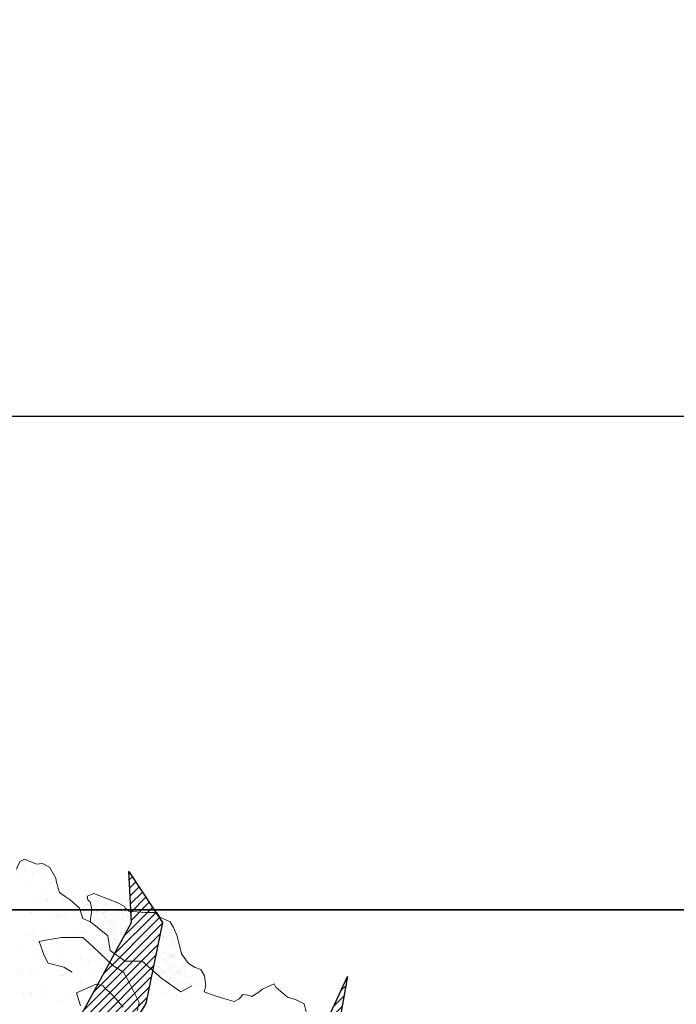
# Model space of a CAD drawing. Units: inches. Extents: x 1986 to 21484, y -1816 to 2016.
# Tile 39 of 85: x 2175 to 2192, y 1898 to 1924. Entities that reach past the tile are written whole.
import ezdxf

# ---------------------------------------------------------------- set-up
doc = ezdxf.new("R2010")
doc.units = ezdxf.units.IN
for name, color, linetype, lineweight in [('A-ANNO-DIMS', 2, 'Continuous', 18), ('C-PROP', 7, 'Continuous', 35), ('L-PLNT', 84, 'Continuous', 13), ('vfolhas', 114, 'Continuous', 5)]:
    doc.layers.add(name, color=color, linetype=linetype, lineweight=lineweight)
doc.layers.add('vfolhas2', color=102, linetype='Continuous')
doc.styles.get("Standard").update_dxf_attribs({"font": 'arial.ttf'})
doc.dimstyles.new('ISO-25', dxfattribs={"dimtxt": 8, "dimasz": 2.5, "dimexe": 1.25, "dimexo": 0.625, "dimtad": 1, "dimdec": 1, "dimlunit": 3, "dimtxsty": 'Standard', "dimcen": 2.5, "dimadec": 0, "dimazin": 0, "dimtfac": 1, "dimtdec": 1, "dimtmove": 0, "dimatfit": 3, "dimfxl": 1, "dimarcsym": 0})

# ---------------------------------------------------------------- blocks, each defined once
blk = doc.blocks.new('*D1')
at = {"layer": 'A-ANNO-DIMS', "color": 0, "lineweight": -2, "transparency": 16777216}
for p, q in [((2042.312, 1901.377), (2042.312, 1914.655)), ((2402.312, 1901.377), (2402.312, 1914.655)), ((2044.812, 1913.405), (2399.812, 1913.405))]:
    blk.add_line(p, q, dxfattribs=at)
at = {"layer": 'A-ANNO-DIMS', "color": 0, "transparency": 16777216}
for points in [[(2044.812, 1913.821), (2044.812, 1912.988), (2042.312, 1913.405)], [(2399.812, 1913.821), (2399.812, 1912.988), (2402.312, 1913.405)]]:
    blk.add_solid(points, dxfattribs=at)
at = {"layer": 'Defpoints', "color": 0, "transparency": 16777216}
for p in [(2402.312, 1913.405), (2042.312, 1900.752), (2402.312, 1900.752)]:
    blk.add_point(p, dxfattribs=at)
at = {"layer": 'A-ANNO-DIMS', "color": 0, "transparency": 16777216, "insert": (2222.312, 1918.117), "char_height": 8, "attachment_point": 5}
blk.add_mtext("30'", dxfattribs=at)
blk = doc.blocks.new('arbusto_PB_verde_grande')
at = {"layer": 'vfolhas'}
h = blk.add_hatch(dxfattribs=at)
h.set_pattern_fill('ANSI31', color=256, scale=0.05, style=0)
h.set_pattern_definition([(45, (-2446.5133113, 50.986076), (-0.004419417382, 0.004419417382), [])])
h.paths.add_polyline_path([(-0.0728, 0.5067), (-0.1808, 0.6506), (-0.2334, 0.6725), (-0.2071, 0.5318), (-0.1078, 0.2501), (0.0263, -0.0393), (0.0003, 0.0905), (0.0082, 0.1624), (-0.0494, 0.2908)])
h.paths.add_polyline_path([(0.099, 0.4193), (0.0937, 0.2657), (0.0791, 0.1881), (0.1551, 0.369), (0.2661, 0.5505), (0.2836, 0.635), (0.2485, 0.6882), (0.2514, 0.635), (0.2018, 0.5443)])
h.paths.add_polyline_path([(0.1229, 0.2407), (0.047, 0.0623), (0.0263, -0.0393), (0.1112, 0.0436), (0.1843, 0.0936), (0.2748, 0.1938), (0.3215, 0.2532), (0.4413, 0.3847), (0.4763, 0.5787), (0.4179, 0.4535), (0.2894, 0.3095)])
h.paths.add_polyline_path([(0.5815, -0.0378), (0.7071, 0.0154), (0.7859, 0.0467), (0.748, 0.0655), (0.6282, 0.0842), (0.526, 0.0905), (0.3974, 0.0436), (0.0263, -0.0393), (0.2573, -0.0315), (0.4383, -0.0347)])
h.paths.add_polyline_path([(0.5202, -0.0365), (0.4383, -0.0347), (0.2573, -0.0315), (0.0263, -0.0393), (0.1796, -0.0852), (0.5377, -0.1317), (0.6954, -0.1536), (0.7859, -0.0785), (0.7041, -0.1004)])
h.paths.add_polyline_path([(0.2719, -0.2193), (0.1492, -0.1411), (0.0263, -0.0393), (0.1579, -0.3101), (0.2952, -0.4258), (0.4179, -0.4916), (0.564, -0.5667), (0.5114, -0.4853), (0.3946, -0.3414)])
h.paths.add_polyline_path([(-0.0582, -0.4759), (-0.0231, -0.6198), (0.047, -0.8013), (0.0849, -0.5979), (0.0791, -0.4071), (0.0353, -0.2538), (0.0263, -0.0393), (-0.0377, -0.26)])
h.paths.add_polyline_path([(-0.2422, 0.1405), (-0.1107, 0.0686), (0.0263, -0.0393), (-0.0423, 0.1087), (-0.2101, 0.2376), (-0.3649, 0.3314), (-0.4787, 0.4034), (-0.543, 0.4629), (-0.4904, 0.3314), (-0.3941, 0.2219)])
at = {"layer": 'vfolhas2'}
for p, q in [((0.2514, 0.635), (0.2485, 0.6882)), ((0.2485, 0.6882), (0.2836, 0.635)), ((0.2018, 0.5443), (0.2514, 0.635)), ((0.2836, 0.635), (0.2661, 0.5505)), ((0.4179, 0.4535), (0.4763, 0.5787)), ((0.4763, 0.5787), (0.4413, 0.3847)), ((0.2661, 0.5505), (0.1551, 0.369))]:
    blk.add_line(p, q, dxfattribs=at)
blk = doc.blocks.new('PLANT-SHRUB')
for p, q in [((2174.858, 1901.798), (2174.94, 1901.995)), ((2174.94, 1901.995), (2175.064, 1902.05)), ((2175.064, 1902.05), (2175.366, 1901.922)), ((2175.366, 1901.922), (2175.526, 1901.936)), ((2175.526, 1901.936), (2175.7, 1901.844)), ((2175.071, 1901.745), (2175.071, 1901.745)), ((2175.279, 1901.717), (2175.279, 1901.717)), ((2175.604, 1901.675), (2175.604, 1901.675)), ((2175.7, 1901.844), (2175.862, 1901.568)), ((2174.953, 1901.579), (2174.953, 1901.579)), ((2175.862, 1901.568), (2175.88, 1901.454)), ((2175.88, 1901.454), (2175.958, 1901.197)), ((2175.095, 1901.383), (2175.095, 1901.383)), ((2175.591, 1901.19), (2175.591, 1901.19)), ((2175.958, 1901.197), (2176.104, 1901.092)), ((2176.668, 1901.106), (2176.842, 1901.17)), ((2176.842, 1901.17), (2177.451, 1900.932)), ((2176.842, 1901.17), (2176.842, 1901.17)), ((2175.423, 1901.083), (2175.423, 1901.083)), ((2175.611, 1900.988), (2175.611, 1900.988)), ((2175.65, 1900.999), (2175.65, 1900.999)), ((2175.724, 1901.066), (2175.724, 1901.066)), ((2176.104, 1901.092), (2176.233, 1901.01)), ((2176.233, 1901.01), (2176.471, 1900.795)), ((2176.686, 1901.005), (2176.668, 1901.106)), ((2176.745, 1900.95), (2176.686, 1901.005)), ((2176.777, 1900.822), (2176.745, 1900.95)), ((2177.273, 1901.034), (2177.273, 1901.034)), ((2177.451, 1900.932), (2177.615, 1900.85)), ((2177.679, 1900.98), (2177.679, 1900.98)), ((2177.912, 1901.079), (2177.912, 1901.079)), ((2175.235, 1900.688), (2175.235, 1900.688)), ((2176.471, 1900.795), (2176.53, 1900.603)), ((2176.755, 1900.52), (2176.777, 1900.69)), ((2176.777, 1900.74), (2176.777, 1900.822)), ((2176.777, 1900.69), (2176.777, 1900.74)), ((2176.837, 1900.684), (2176.837, 1900.684)), ((2176.911, 1900.722), (2176.911, 1900.722)), ((2176.92, 1900.673), (2176.92, 1900.673)), ((2176.926, 1900.715), (2176.926, 1900.715)), ((2176.966, 1900.738), (2176.966, 1900.738)), ((2177.05, 1900.656), (2177.05, 1900.656)), ((2177.07, 1900.868), (2177.07, 1900.868)), ((2177.082, 1900.68), (2177.082, 1900.68)), ((2177.1, 1900.895), (2177.1, 1900.895)), ((2177.149, 1900.723), (2177.149, 1900.723)), ((2177.182, 1900.887), (2177.182, 1900.887)), ((2177.375, 1900.74), (2177.375, 1900.74)), ((2177.392, 1900.878), (2177.392, 1900.878)), ((2177.551, 1900.728), (2177.551, 1900.728)), ((2177.58, 1900.755), (2177.58, 1900.755)), ((2177.58, 1900.679), (2177.58, 1900.679)), ((2177.615, 1900.85), (2177.643, 1900.799)), ((2177.643, 1900.799), (2177.739, 1900.722)), ((2177.647, 1900.722), (2177.647, 1900.722)), ((2177.739, 1900.722), (2178.158, 1900.688)), ((2178.078, 1900.678), (2178.078, 1900.678)), ((2178.158, 1900.688), (2178.451, 1900.684)), ((2178.158, 1900.688), (2178.158, 1900.688)), ((2178.451, 1900.684), (2178.533, 1900.565)), ((2175.07, 1900.613), (2175.07, 1900.613)), ((2175.253, 1900.634), (2175.253, 1900.634)), ((2175.778, 1900.617), (2175.778, 1900.617)), ((2175.875, 1900.576), (2175.875, 1900.576)), ((2175.986, 1900.59), (2175.986, 1900.59)), ((2176.092, 1900.618), (2176.092, 1900.618)), ((2176.311, 1900.547), (2176.311, 1900.547)), ((2176.53, 1900.603), (2176.553, 1900.534)), ((2176.553, 1900.534), (2176.755, 1900.447)), ((2176.755, 1900.447), (2176.755, 1900.52)), ((2176.755, 1900.447), (2177.201, 1900.084)), ((2176.765, 1900.478), (2176.765, 1900.478)), ((2176.772, 1900.595), (2176.772, 1900.595)), ((2176.852, 1900.648), (2176.852, 1900.648)), ((2176.854, 1900.475), (2176.854, 1900.475)), ((2176.956, 1900.43), (2176.956, 1900.43)), ((2177.062, 1900.448), (2177.062, 1900.448)), ((2177.12, 1900.574), (2177.12, 1900.574)), ((2177.172, 1900.579), (2177.172, 1900.579)), ((2177.172, 1900.579), (2177.172, 1900.579)), ((2177.223, 1900.428), (2177.223, 1900.428)), ((2177.253, 1900.455), (2177.253, 1900.455)), ((2177.263, 1900.477), (2177.263, 1900.477)), ((2177.268, 1900.628), (2177.268, 1900.628)), ((2177.351, 1900.617), (2177.351, 1900.617)), ((2177.365, 1900.431), (2177.365, 1900.431)), ((2177.387, 1900.405), (2177.387, 1900.405)), ((2177.392, 1900.582), (2177.392, 1900.582)), ((2177.481, 1900.6), (2177.481, 1900.6)), ((2177.59, 1900.574), (2177.59, 1900.574)), ((2177.698, 1900.571), (2177.698, 1900.571)), ((2177.761, 1900.476), (2177.761, 1900.476)), ((2177.781, 1900.56), (2177.781, 1900.56)), ((2177.797, 1900.416), (2177.797, 1900.416)), ((2177.872, 1900.442), (2177.872, 1900.442)), ((2177.911, 1900.543), (2177.911, 1900.543)), ((2177.999, 1900.576), (2177.999, 1900.576)), ((2178.032, 1900.588), (2178.032, 1900.588)), ((2178.061, 1900.615), (2178.061, 1900.615)), ((2178.128, 1900.514), (2178.128, 1900.514)), ((2178.211, 1900.504), (2178.211, 1900.504)), ((2178.215, 1900.411), (2178.215, 1900.411)), ((2178.218, 1900.566), (2178.218, 1900.566)), ((2178.259, 1900.475), (2178.259, 1900.475)), ((2178.341, 1900.486), (2178.341, 1900.486)), ((2178.364, 1900.572), (2178.364, 1900.572)), ((2178.512, 1900.447), (2178.512, 1900.447)), ((2178.533, 1900.565), (2178.799, 1900.441)), ((2178.542, 1900.474), (2178.542, 1900.474)), ((2178.558, 1900.458), (2178.558, 1900.458)), ((2178.624, 1900.413), (2178.624, 1900.413)), ((2178.642, 1900.447), (2178.642, 1900.447)), ((2178.799, 1900.441), (2178.877, 1900.299)), ((2175.268, 1900.19), (2175.268, 1900.19)), ((2175.585, 1900.218), (2175.585, 1900.218)), ((2176.454, 1900.283), (2176.454, 1900.283)), ((2176.513, 1900.187), (2176.513, 1900.187)), ((2176.632, 1900.205), (2176.632, 1900.205)), ((2177.02, 1900.323), (2177.02, 1900.323)), ((2177.064, 1900.282), (2177.064, 1900.282)), ((2177.12, 1900.233), (2177.12, 1900.233)), ((2177.162, 1900.271), (2177.162, 1900.271)), ((2177.203, 1900.222), (2177.203, 1900.222)), ((2177.333, 1900.205), (2177.333, 1900.205)), ((2177.451, 1900.279), (2177.451, 1900.279)), ((2177.518, 1900.322), (2177.518, 1900.322)), ((2177.55, 1900.177), (2177.55, 1900.177)), ((2177.58, 1900.266), (2177.58, 1900.266)), ((2177.634, 1900.166), (2177.634, 1900.166)), ((2177.654, 1900.21), (2177.654, 1900.21)), ((2177.704, 1900.287), (2177.704, 1900.287)), ((2177.733, 1900.314), (2177.733, 1900.314)), ((2177.758, 1900.185), (2177.758, 1900.185)), ((2177.764, 1900.149), (2177.764, 1900.149)), ((2177.93, 1900.334), (2177.93, 1900.334)), ((2177.949, 1900.278), (2177.949, 1900.278)), ((2177.989, 1900.268), (2177.989, 1900.268)), ((2178.016, 1900.321), (2178.016, 1900.321)), ((2178.053, 1900.297), (2178.053, 1900.297)), ((2178.127, 1900.365), (2178.127, 1900.365)), ((2178.138, 1900.306), (2178.138, 1900.306)), ((2178.184, 1900.147), (2178.184, 1900.147)), ((2178.214, 1900.174), (2178.214, 1900.174)), ((2178.353, 1900.301), (2178.353, 1900.301)), ((2178.421, 1900.252), (2178.421, 1900.252)), ((2178.446, 1900.277), (2178.446, 1900.277)), ((2178.463, 1900.263), (2178.463, 1900.263)), ((2178.514, 1900.32), (2178.514, 1900.32)), ((2178.733, 1900.171), (2178.733, 1900.171)), ((2178.834, 1900.161), (2178.834, 1900.161)), ((2178.84, 1900.247), (2178.84, 1900.247)), ((2178.877, 1900.299), (2178.973, 1900.08)), ((2175.1, 1900.082), (2175.1, 1900.082)), ((2175.437, 1899.94), (2175.652, 1899.983)), ((2175.566, 1899.582), (2175.437, 1899.94)), ((2175.652, 1899.983), (2176.011, 1900.041)), ((2176.011, 1900.041), (2176.254, 1900.041)), ((2176.033, 1899.897), (2176.033, 1899.897)), ((2176.106, 1899.965), (2176.106, 1899.965)), ((2176.254, 1900.041), (2176.556, 1900.041)), ((2176.344, 1900.08), (2176.344, 1900.08)), ((2176.556, 1900.041), (2176.814, 1899.811)), ((2177.201, 1900.084), (2177.258, 1899.711)), ((2177.355, 1900.123), (2177.355, 1900.123)), ((2177.376, 1899.987), (2177.376, 1899.987)), ((2177.389, 1899.921), (2177.389, 1899.921)), ((2177.406, 1900.014), (2177.406, 1900.014)), ((2177.545, 1900.142), (2177.545, 1900.142)), ((2177.57, 1899.958), (2177.57, 1899.958)), ((2177.589, 1900.078), (2177.589, 1900.078)), ((2177.632, 1900.076), (2177.632, 1900.076)), ((2177.656, 1899.933), (2177.656, 1899.933)), ((2177.786, 1900.108), (2177.786, 1900.108)), ((2177.887, 1899.92), (2177.887, 1899.92)), ((2177.979, 1899.96), (2177.979, 1899.96)), ((2177.981, 1900.12), (2177.981, 1900.12)), ((2178.025, 1900.001), (2178.025, 1900.001)), ((2178.064, 1900.109), (2178.064, 1900.109)), ((2178.13, 1900.075), (2178.13, 1900.075)), ((2178.194, 1900.092), (2178.194, 1900.092)), ((2178.205, 1900.103), (2178.205, 1900.103)), ((2178.385, 1899.92), (2178.385, 1899.92)), ((2178.411, 1900.063), (2178.411, 1900.063)), ((2178.411, 1899.944), (2178.411, 1899.944)), ((2178.494, 1900.052), (2178.494, 1900.052)), ((2178.614, 1900.105), (2178.614, 1900.105)), ((2178.624, 1900.035), (2178.624, 1900.035)), ((2178.627, 1900.074), (2178.627, 1900.074)), ((2178.665, 1900.007), (2178.665, 1900.007)), ((2178.694, 1900.034), (2178.694, 1900.034)), ((2178.83, 1899.939), (2178.83, 1899.939)), ((2178.834, 1900.075), (2178.834, 1900.075)), ((2178.841, 1900.007), (2178.841, 1900.007)), ((2178.883, 1899.919), (2178.883, 1899.919)), ((2178.925, 1899.996), (2178.925, 1899.996)), ((2178.973, 1900.08), (2179.083, 1899.622)), ((2175.045, 1899.843), (2175.045, 1899.843)), ((2176.067, 1899.848), (2176.067, 1899.848)), ((2176.814, 1899.811), (2177.33, 1899.324)), ((2176.814, 1899.811), (2176.814, 1899.811)), ((2177.147, 1899.809), (2177.147, 1899.809)), ((2177.258, 1899.711), (2177.646, 1899.439)), ((2177.322, 1899.878), (2177.322, 1899.878)), ((2177.345, 1899.815), (2177.345, 1899.815)), ((2177.403, 1899.782), (2177.403, 1899.782)), ((2177.486, 1899.771), (2177.486, 1899.771)), ((2177.503, 1899.676), (2177.503, 1899.676)), ((2177.56, 1899.65), (2177.56, 1899.65)), ((2177.616, 1899.754), (2177.616, 1899.754)), ((2177.698, 1899.701), (2177.698, 1899.701)), ((2177.776, 1899.8), (2177.776, 1899.8)), ((2177.819, 1899.878), (2177.819, 1899.878)), ((2177.833, 1899.725), (2177.833, 1899.725)), ((2177.857, 1899.847), (2177.857, 1899.847)), ((2177.886, 1899.874), (2177.886, 1899.874)), ((2177.917, 1899.714), (2177.917, 1899.714)), ((2177.969, 1899.652), (2177.969, 1899.652)), ((2178, 1899.675), (2178, 1899.675)), ((2178.047, 1899.697), (2178.047, 1899.697)), ((2178.193, 1899.796), (2178.193, 1899.796)), ((2178.195, 1899.795), (2178.195, 1899.795)), ((2178.264, 1899.669), (2178.264, 1899.669)), ((2178.317, 1899.877), (2178.317, 1899.877)), ((2178.337, 1899.706), (2178.337, 1899.706)), ((2178.347, 1899.658), (2178.347, 1899.658)), ((2178.367, 1899.733), (2178.367, 1899.733)), ((2178.477, 1899.641), (2178.477, 1899.641)), ((2178.498, 1899.674), (2178.498, 1899.674)), ((2178.506, 1899.861), (2178.506, 1899.861)), ((2178.604, 1899.796), (2178.604, 1899.796)), ((2178.815, 1899.876), (2178.815, 1899.876)), ((2178.986, 1899.721), (2178.986, 1899.721)), ((2178.996, 1899.673), (2178.996, 1899.673)), ((2179.036, 1899.781), (2179.036, 1899.781)), ((2175.41, 1899.631), (2175.41, 1899.631)), ((2175.552, 1899.575), (2175.552, 1899.575)), ((2175.56, 1899.448), (2175.56, 1899.448)), ((2175.666, 1899.382), (2175.566, 1899.582)), ((2175.618, 1899.603), (2175.618, 1899.603)), ((2175.635, 1899.533), (2175.635, 1899.533)), ((2175.942, 1899.56), (2175.942, 1899.56)), ((2176.485, 1899.489), (2176.485, 1899.489)), ((2176.606, 1899.435), (2176.606, 1899.435)), ((2176.693, 1899.462), (2176.693, 1899.462)), ((2176.797, 1899.573), (2176.797, 1899.573)), ((2177.018, 1899.419), (2177.018, 1899.419)), ((2177.234, 1899.546), (2177.234, 1899.546)), ((2177.308, 1899.614), (2177.308, 1899.614)), ((2177.529, 1899.546), (2177.529, 1899.546)), ((2177.559, 1899.573), (2177.559, 1899.573)), ((2177.629, 1899.439), (2177.629, 1899.439)), ((2177.646, 1899.439), (2178.076, 1899.439)), ((2177.69, 1899.477), (2177.69, 1899.477)), ((2177.758, 1899.52), (2177.758, 1899.52)), ((2177.766, 1899.492), (2177.766, 1899.492)), ((2178.041, 1899.571), (2178.041, 1899.571)), ((2178.076, 1899.439), (2178.578, 1898.995)), ((2178.076, 1899.439), (2178.076, 1899.439)), ((2178.178, 1899.561), (2178.178, 1899.561)), ((2178.185, 1899.486), (2178.185, 1899.486)), ((2178.188, 1899.476), (2178.188, 1899.476)), ((2178.256, 1899.519), (2178.256, 1899.519)), ((2178.401, 1899.636), (2178.401, 1899.636)), ((2178.594, 1899.488), (2178.594, 1899.488)), ((2178.659, 1899.42), (2178.659, 1899.42)), ((2178.686, 1899.475), (2178.686, 1899.475)), ((2178.694, 1899.612), (2178.694, 1899.612)), ((2178.708, 1899.401), (2178.708, 1899.401)), ((2178.753, 1899.518), (2178.753, 1899.518)), ((2178.777, 1899.601), (2178.777, 1899.601)), ((2178.818, 1899.566), (2178.818, 1899.566)), ((2178.819, 1899.631), (2178.819, 1899.631)), ((2178.847, 1899.593), (2178.847, 1899.593)), ((2178.857, 1899.582), (2178.857, 1899.582)), ((2178.907, 1899.584), (2178.907, 1899.584)), ((2179.026, 1899.473), (2179.026, 1899.473)), ((2179.083, 1899.622), (2179.266, 1899.378)), ((2179.124, 1899.555), (2179.124, 1899.555)), ((2179.184, 1899.474), (2179.184, 1899.474)), ((2174.945, 1899.189), (2174.945, 1899.189)), ((2175.214, 1899.147), (2175.214, 1899.147)), ((2175.287, 1899.214), (2175.287, 1899.214)), ((2176.068, 1899.281), (2175.666, 1899.382)), ((2176.283, 1899.152), (2176.068, 1899.281)), ((2176.19, 1899.187), (2176.19, 1899.187)), ((2176.836, 1899.182), (2176.836, 1899.182)), ((2177.33, 1899.324), (2177.603, 1899.152)), ((2177.435, 1899.184), (2177.435, 1899.184)), ((2177.561, 1899.347), (2177.561, 1899.347)), ((2177.603, 1899.152), (2177.717, 1898.937)), ((2177.769, 1899.32), (2177.769, 1899.32)), ((2178.094, 1899.277), (2178.094, 1899.277)), ((2178.329, 1899.246), (2178.329, 1899.246)), ((2178.369, 1899.274), (2178.369, 1899.274)), ((2178.391, 1899.328), (2178.391, 1899.328)), ((2178.436, 1899.196), (2178.436, 1899.196)), ((2178.49, 1899.266), (2178.49, 1899.266)), ((2178.509, 1899.263), (2178.509, 1899.263)), ((2178.52, 1899.293), (2178.52, 1899.293)), ((2178.547, 1899.218), (2178.547, 1899.218)), ((2178.584, 1899.18), (2178.584, 1899.18)), ((2178.63, 1899.207), (2178.63, 1899.207)), ((2178.637, 1899.206), (2178.637, 1899.206)), ((2178.679, 1899.182), (2178.679, 1899.182)), ((2178.76, 1899.19), (2178.76, 1899.19)), ((2178.809, 1899.323), (2178.809, 1899.323)), ((2178.845, 1899.178), (2178.845, 1899.178)), ((2178.867, 1899.273), (2178.867, 1899.273)), ((2178.977, 1899.161), (2178.977, 1899.161)), ((2179, 1899.153), (2179, 1899.153)), ((2179.015, 1899.165), (2179.015, 1899.165)), ((2179.06, 1899.15), (2179.06, 1899.15)), ((2179.139, 1899.28), (2179.139, 1899.28)), ((2179.17, 1899.136), (2179.17, 1899.136)), ((2179.218, 1899.325), (2179.218, 1899.325)), ((2179.266, 1899.378), (2179.436, 1899.277)), ((2179.365, 1899.272), (2179.365, 1899.272)), ((2179.436, 1899.277), (2179.582, 1899.222)), ((2179.582, 1899.222), (2179.674, 1899.057)), ((2175.02, 1899.073), (2175.02, 1899.073)), ((2176.022, 1899.079), (2176.022, 1899.079)), ((2176.042, 1899.078), (2176.042, 1899.078)), ((2177.122, 1899.039), (2177.122, 1899.039)), ((2177.266, 1899.077), (2177.266, 1899.077)), ((2177.717, 1898.937), (2178.004, 1898.378)), ((2177.717, 1898.937), (2177.717, 1898.937)), ((2178.168, 1899.026), (2178.168, 1899.026)), ((2178.511, 1899.075), (2178.511, 1899.075)), ((2178.557, 1899.075), (2178.557, 1899.075)), ((2178.578, 1898.995), (2179.065, 1898.651)), ((2178.624, 1899.118), (2178.624, 1899.118)), ((2178.799, 1899.015), (2178.799, 1899.015)), ((2178.812, 1898.98), (2178.812, 1898.98)), ((2178.971, 1899.126), (2178.971, 1899.126)), ((2179.055, 1899.074), (2179.055, 1899.074)), ((2179.122, 1899.117), (2179.122, 1899.117)), ((2179.19, 1899.133), (2179.19, 1899.133)), ((2179.19, 1899.031), (2179.19, 1899.031)), ((2179.208, 1899.017), (2179.208, 1899.017)), ((2179.407, 1899.104), (2179.407, 1899.104)), ((2179.451, 1898.985), (2179.451, 1898.985)), ((2179.674, 1899.057), (2179.711, 1898.806)), ((2175.041, 1898.644), (2175.041, 1898.644)), ((2175.535, 1898.678), (2175.535, 1898.678)), ((2176.9, 1898.851), (2176.398, 1898.622)), ((2176.415, 1898.796), (2176.415, 1898.796)), ((2176.489, 1898.863), (2176.489, 1898.863)), ((2176.581, 1898.664), (2176.581, 1898.664)), ((2176.9, 1898.851), (2176.9, 1898.851)), ((2177.072, 1898.808), (2176.9, 1898.851)), ((2177.344, 1898.536), (2177.072, 1898.808)), ((2177.604, 1898.669), (2177.604, 1898.669)), ((2178.038, 1898.831), (2178.038, 1898.831)), ((2178.683, 1898.631), (2178.683, 1898.631)), ((2178.993, 1898.717), (2178.993, 1898.717)), ((2179.005, 1898.857), (2179.005, 1898.857)), ((2179.043, 1898.738), (2179.043, 1898.738)), ((2179.065, 1898.651), (2179.352, 1898.808)), ((2179.065, 1898.651), (2179.065, 1898.651)), ((2179.124, 1898.685), (2179.124, 1898.685)), ((2179.153, 1898.712), (2179.153, 1898.712)), ((2179.236, 1898.871), (2179.236, 1898.871)), ((2179.292, 1898.839), (2179.292, 1898.839)), ((2179.424, 1898.851), (2179.424, 1898.851)), ((2179.711, 1898.806), (2179.665, 1898.65)), ((2179.665, 1898.65), (2179.926, 1898.554)), ((2181.045, 1898.621), (2181.164, 1898.718)), ((2181.164, 1898.718), (2181.466, 1898.859)), ((2181.164, 1898.718), (2181.164, 1898.718)), ((2181.466, 1898.859), (2181.507, 1898.768)), ((2181.466, 1898.859), (2181.466, 1898.859)), ((2181.507, 1898.768), (2181.8, 1898.516)), ((2175.229, 1898.574), (2175.229, 1898.574)), ((2175.249, 1898.617), (2175.249, 1898.617)), ((2175.574, 1898.574), (2175.574, 1898.574)), ((2176.017, 1898.431), (2176.017, 1898.431)), ((2176.117, 1898.503), (2176.117, 1898.503)), ((2176.325, 1898.475), (2176.325, 1898.475)), ((2176.398, 1898.622), (2176.498, 1898.292)), ((2176.398, 1898.622), (2176.398, 1898.622)), ((2176.474, 1898.572), (2176.474, 1898.572)), ((2176.65, 1898.433), (2176.65, 1898.433)), ((2177.594, 1898.258), (2177.344, 1898.536)), ((2177.616, 1898.445), (2177.616, 1898.445)), ((2177.69, 1898.513), (2177.69, 1898.513)), ((2177.719, 1898.57), (2177.719, 1898.57)), ((2178.004, 1898.378), (2177.947, 1898.163)), ((2178.963, 1898.568), (2178.963, 1898.568)), ((2179.239, 1898.48), (2179.239, 1898.48)), ((2179.729, 1898.617), (2179.729, 1898.617)), ((2179.926, 1898.554), (2180.136, 1898.49)), ((2180.136, 1898.49), (2180.44, 1898.406)), ((2180.136, 1898.49), (2180.136, 1898.49)), ((2180.44, 1898.406), (2180.564, 1898.47)), ((2180.564, 1898.47), (2180.669, 1898.58)), ((2180.669, 1898.58), (2180.788, 1898.567)), ((2180.788, 1898.567), (2180.889, 1898.53)), ((2180.839, 1898.494), (2180.839, 1898.494)), ((2180.889, 1898.53), (2181.045, 1898.621)), ((2180.912, 1898.562), (2180.912, 1898.562)), ((2181.8, 1898.516), (2182.011, 1898.452)), ((2182.011, 1898.452), (2182.235, 1898.347)), ((2177.193, 1898.361), (2177.193, 1898.361)), ((2177.401, 1898.334), (2177.401, 1898.334)), ((2182.235, 1898.347), (2182.286, 1898.137))]:
    blk.add_line(p, q)

msp = doc.modelspace()

# ---------------------------------------------------------------- linework, layer by layer
at = {"layer": 'C-PROP'}
msp.add_lwpolyline([(2042.312, 1900.752), (2402.312, 1900.752), (2402.312, 1066.752), (2042.312, 1066.752)], close=True, dxfattribs=at)

# ---------------------------------------------------------------- block references
at = {"layer": 'L-PLNT'}
msp.add_blockref('PLANT-SHRUB', (0, 0), dxfattribs=at)
at = {"layer": 'L-PLNT', "xscale": 24.60366729364114, "yscale": 24.60366729364114, "zscale": 24.60366729364114}
msp.add_blockref('arbusto_PB_verde_grande', (2171.623, 1884.805), dxfattribs=at)

# ---------------------------------------------------------------- dimensions: what is measured, and where the dimension line sits
at = {"layer": 'A-ANNO-DIMS'}
dim = msp.add_linear_dim(base=(2402.312, 1913.405), p1=(2042.312, 1900.752), p2=(2402.312, 1900.752), dimstyle='ISO-25', override={"dimclrd": 0, "dimclre": 0, "dimclrt": 0}, dxfattribs=at)
dim.commit()
dim.dimension.update_dxf_attribs({"geometry": '*D1', "text_midpoint": (2222.312, 1918.117)})

doc.saveas('drawing.dxf')
